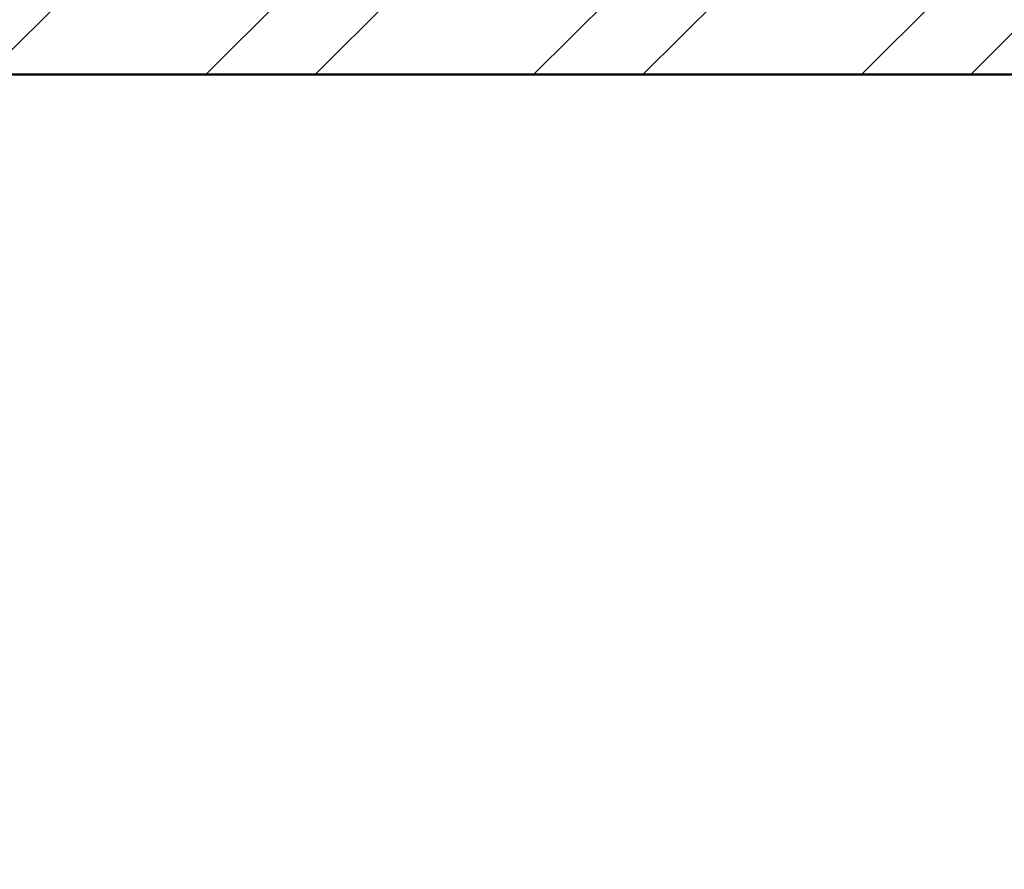
# Model space of a CAD drawing. Units: inches. Extents: x 963 to 2075, y 289 to 2657.
# Tile 77 of 98: x 1426 to 1467, y 2290 to 2325. Entities that reach past the tile are written whole.
import ezdxf

# ---------------------------------------------------------------- set-up
doc = ezdxf.new("R2010")
doc.units = ezdxf.units.IN
doc.layers.add('A-WALL', color=7, linetype='Continuous', lineweight=50)
doc.layers.add('A-WALL-PATT', color=8, linetype='Continuous', lineweight=13)

msp = doc.modelspace()

# ---------------------------------------------------------------- hatches: boundary and pattern name
at = {"layer": 'A-WALL-PATT'}
h = msp.add_hatch(dxfattribs=at)
h.set_pattern_fill('ANSI32', color=256)
h.paths.add_polyline_path([(1296.922, 2558.318), (1203.922, 2558.318), (1203.922, 2493.818), (1191.533, 2493.818), (1191.533, 2489.318), (1211.063, 2489.318), (1211.063, 2492.02), (1211.063, 2493.818), (1208.422, 2493.818), (1208.422, 2553.818), (1292.422, 2553.818), (1292.422, 2538.863), (1296.922, 2538.863)])
h.paths.add_polyline_path([(1442.422, 2558.318), (1349.422, 2558.318), (1349.422, 2538.943), (1353.922, 2538.943), (1353.922, 2553.818), (1437.922, 2553.818), (1437.922, 2493.818), (1434.542, 2493.818), (1434.542, 2489.318), (1448.311, 2489.318), (1448.311, 2491.568), (1448.311, 2493.818), (1442.422, 2493.818)])
h.paths.add_polyline_path([(1415.554, 2491.568), (1415.554, 2493.818), (1340.941, 2493.818), (1340.941, 2489.318), (1371.922, 2489.318), (1371.922, 2378.318), (1367.596, 2378.318), (1367.596, 2373.818), (1371.922, 2373.818), (1371.922, 2355.185), (1376.422, 2355.185), (1376.422, 2489.318), (1415.554, 2489.318)])
h.paths.add_polyline_path([(1304.941, 2491.568), (1304.941, 2493.818), (1296.922, 2493.818), (1296.922, 2514.863), (1292.422, 2514.863), (1292.422, 2493.818), (1232.808, 2493.818), (1232.808, 2489.318), (1256.422, 2489.318), (1256.422, 2327.318), (1253.714, 2327.318), (1253.714, 2322.818), (1328.422, 2322.818), (1328.422, 2331.147), (1323.922, 2331.147), (1323.922, 2327.318), (1260.922, 2327.318), (1260.922, 2373.818), (1323.922, 2373.818), (1323.922, 2357.812), (1328.422, 2357.812), (1328.422, 2373.818), (1346.007, 2373.818), (1346.007, 2376.068), (1346.007, 2378.318), (1260.922, 2378.318), (1260.922, 2489.318), (1304.941, 2489.318)])
h.paths.add_polyline_path([(1226.654, 2327.318), (1124.422, 2327.318), (1124.422, 2347.447), (1119.922, 2347.447), (1119.922, 2322.818), (1163.422, 2322.818), (1163.422, 2305.435), (1165.672, 2305.435), (1167.922, 2305.435), (1167.922, 2322.818), (1226.654, 2322.818), (1226.654, 2325.068)])
h.paths.add_polyline_path([(1095.922, 2489.318), (1124.422, 2489.318), (1131.533, 2489.318), (1131.533, 2491.568), (1131.533, 2493.818), (1119.922, 2493.818), (1091.422, 2493.818), (1091.422, 2417.318), (1095.922, 2417.318), (1119.922, 2417.318), (1119.922, 2407.447), (1124.422, 2407.447), (1124.422, 2421.818), (1095.922, 2421.818)])
h.paths.add_polyline_path([(1512.922, 2558.318), (1508.422, 2558.318), (1508.422, 2493.818), (1503.401, 2493.818), (1503.401, 2489.318), (1508.422, 2489.318), (1508.422, 2327.318), (1376.422, 2327.318), (1376.422, 2330.273), (1371.922, 2330.273), (1371.922, 2298.744), (1376.422, 2298.744), (1376.422, 2322.818), (1508.422, 2322.818), (1508.422, 2165.318), (1504.255, 2165.318), (1504.255, 2160.818), (1508.422, 2160.818), (1508.422, 2108.318), (1512.922, 2108.318), (1512.922, 2160.818), (1516.182, 2160.818), (1516.182, 2163.068), (1516.182, 2165.318), (1512.922, 2165.318), (1512.922, 2322.818), (1644.922, 2322.818), (1644.922, 2298.744), (1649.422, 2298.744), (1649.422, 2322.818), (1649.422, 2330.944), (1647.172, 2330.944), (1644.922, 2330.944), (1644.922, 2327.318), (1512.922, 2327.318), (1512.922, 2489.318), (1516.759, 2489.318), (1516.759, 2491.568), (1516.759, 2493.818), (1512.922, 2493.818)])
h.paths.add_polyline_path([(1671.922, 2558.318), (1578.922, 2558.318), (1578.922, 2493.818), (1573.526, 2493.818), (1573.526, 2489.318), (1586.537, 2489.318), (1586.537, 2491.568), (1586.537, 2493.818), (1583.422, 2493.818), (1583.422, 2553.818), (1667.422, 2553.818), (1667.422, 2541.109), (1671.922, 2541.109)])
h.paths.add_polyline_path([(1681.257, 2493.818), (1671.922, 2493.818), (1671.922, 2517.109), (1667.422, 2517.109), (1667.422, 2493.818), (1610.218, 2493.818), (1610.218, 2489.318), (1644.922, 2489.318), (1644.922, 2357.865), (1649.422, 2357.865), (1649.422, 2373.818), (1652.203, 2373.818), (1652.203, 2375.827), (1652.203, 2378.318), (1649.422, 2378.318), (1649.422, 2489.318), (1681.257, 2489.318), (1681.257, 2491.568)])
h.paths.add_polyline_path([(1821.922, 2558.318), (1728.922, 2558.318), (1728.922, 2541), (1733.422, 2541), (1733.422, 2553.818), (1817.422, 2553.818), (1817.422, 2493.818), (1813.507, 2493.818), (1813.507, 2489.318), (1830.078, 2489.318), (1830.078, 2491.568), (1830.078, 2493.818), (1821.922, 2493.818)])
h.paths.add_polyline_path([(1794.244, 2493.818), (1717.257, 2493.818), (1717.257, 2489.318), (1760.422, 2489.318), (1760.422, 2378.318), (1674.401, 2378.318), (1674.401, 2373.818), (1692.922, 2373.818), (1692.922, 2356.954), (1697.422, 2356.954), (1697.422, 2373.818), (1760.422, 2373.818), (1760.422, 2327.318), (1697.422, 2327.318), (1697.422, 2333.341), (1692.922, 2333.341), (1692.922, 2322.818), (1768.037, 2322.818), (1768.037, 2325.068), (1768.037, 2327.318), (1764.922, 2327.318), (1764.922, 2489.318), (1794.244, 2489.318)])
h.paths.add_polyline_path([(1733.422, 2517), (1728.922, 2517), (1728.922, 2493.818), (1733.422, 2493.818)], flags=17)
h.paths.add_polyline_path([(1929.922, 2493.818), (1890.078, 2493.818), (1890.078, 2489.318), (1896.922, 2489.318), (1925.422, 2489.318), (1925.422, 2421.818), (1896.922, 2421.818), (1896.922, 2408.318), (1901.422, 2408.318), (1901.422, 2417.318), (1925.422, 2417.318), (1929.922, 2417.318)])
h.paths.add_polyline_path([(1901.422, 2348.318), (1896.922, 2348.318), (1896.922, 2327.318), (1800.423, 2327.318), (1800.423, 2322.818), (1853.422, 2322.818), (1853.422, 2309.453), (1857.922, 2309.453), (1857.922, 2322.818), (1901.422, 2322.818)])
h.paths.add_polyline_path([(1857.922, 2249.453), (1853.422, 2249.453), (1853.422, 2214.818), (1686.309, 2214.818), (1686.309, 2210.318), (1853.422, 2210.318), (1853.422, 2202.134), (1857.922, 2202.134), (1857.922, 2210.318)])
h.paths.add_polyline_path([(1857.922, 2142.134), (1853.422, 2142.134), (1853.422, 2115.422), (1841.422, 2115.422), (1841.422, 2088.531), (1841.422, 2046.949), (1845.922, 2046.949), (1845.922, 2110.922), (1905.922, 2110.922), (1905.922, 2092.517), (1910.422, 2092.517), (1910.422, 2115.422), (1857.922, 2115.422)])
h.paths.add_polyline_path([(1532.436, 1482.342), (1573.456, 1482.342), (1573.456, 1501), (1532.436, 1501)], flags=9)
h.paths.add_polyline_path([(1438.658, 1486.302), (1479.678, 1486.302), (1479.678, 1504.96), (1438.658, 1504.96)], flags=9)
h.paths.add_polyline_path([(1411.215, 1365.308), (1659.139, 1365.308), (1659.139, 1402.401), (1411.215, 1402.401)], flags=9)
h.paths.add_polyline_path([(1185.671, 2296.298), (1248.16, 2296.298), (1248.16, 2314.955), (1185.671, 2314.955)], flags=9)
h.paths.add_polyline_path([(1177.31, 2187.35), (1216.15, 2187.35), (1216.15, 2206.007), (1177.31, 2206.007)], flags=9)
h.paths.add_polyline_path([(1295.101, 1602.083), (1328.26, 1602.083), (1328.26, 1620.741), (1295.101, 1620.741)], flags=9)
h.paths.add_polyline_path([(1525.126, 2005.99), (1558.39, 2005.99), (1558.39, 2024.648), (1525.126, 2024.648)], flags=9)
h.paths.add_polyline_path([(1459.606, 1977.125), (1472.195, 1977.125), (1472.195, 1987.429), (1459.606, 1987.429)], flags=9)
h.paths.add_polyline_path([(1467.815, 2053.676), (1480.018, 2053.676), (1480.018, 2063.979), (1467.815, 2063.979)], flags=9)
h.paths.add_polyline_path([(1555.184, 2119.02), (1584.563, 2119.02), (1584.563, 2137.678), (1555.184, 2137.678)], flags=25)
h.paths.add_polyline_path([(1405.389, 2115.291), (1444.478, 2115.291), (1444.478, 2133.948), (1405.389, 2133.948)], flags=25)
h.paths.add_polyline_path([(1698.482, 2004.259), (1727.695, 2004.259), (1727.695, 2022.916), (1698.482, 2022.916)], flags=9)
h.paths.add_polyline_path([(1612.158, 1972.855), (1629.016, 1972.855), (1629.016, 1983.159), (1612.158, 1983.159)], flags=9)
h.paths.add_polyline_path([(1608.289, 2060.036), (1625.147, 2060.036), (1625.147, 2070.34), (1608.289, 2070.34)], flags=9)
h.paths.add_polyline_path([(1527.954, 1684.402), (1566.795, 1684.402), (1566.795, 1703.06), (1527.954, 1703.06)], flags=9)
h.paths.add_polyline_path([(1422.792, 1683.59), (1461.633, 1683.59), (1461.633, 1702.247), (1422.792, 1702.247)], flags=9)
h.paths.add_polyline_path([(1531.262, 1732.459), (1574.015, 1732.459), (1574.015, 1751.116), (1531.262, 1751.116)], flags=9)
h.paths.add_polyline_path([(1402.872, 1732.845), (1439.799, 1732.845), (1439.799, 1751.502), (1402.872, 1751.502)], flags=9)
h.paths.add_polyline_path([(1243.122, 1923.132), (1281.962, 1923.132), (1281.962, 1941.79), (1243.122, 1941.79)], flags=9)
h.paths.add_polyline_path([(1181.752, 1792.268), (1244.241, 1792.268), (1244.241, 1810.926), (1181.752, 1810.926)], flags=9)
h.paths.add_polyline_path([(1265.822, 1670.3), (1316.071, 1670.3), (1316.071, 1688.957), (1265.822, 1688.957)], flags=9)
h.paths.add_polyline_path([(1140.263, 1676.054), (1179.104, 1676.054), (1179.104, 1694.711), (1140.263, 1694.711)], flags=9)
h.paths.add_polyline_path([(1107.49, 1490.889), (1143.374, 1490.889), (1143.374, 1509.546), (1107.49, 1509.546)], flags=9)
h.paths.add_polyline_path([(1217.584, 1483.899), (1246.741, 1483.899), (1246.741, 1502.556), (1217.584, 1502.556)], flags=9)
h.paths.add_polyline_path([(1389.21, 1486.919), (1418.367, 1486.919), (1418.367, 1505.576), (1389.21, 1505.576)], flags=9)
h.paths.add_polyline_path([(1672.208, 1602.083), (1705.366, 1602.083), (1705.366, 1620.741), (1672.208, 1620.741)], flags=9)
h.paths.add_polyline_path([(1752.082, 1522.638), (1781.24, 1522.638), (1781.24, 1541.295), (1752.082, 1541.295)], flags=9)
h.paths.add_polyline_path([(1848.275, 1491.26), (1884.158, 1491.26), (1884.158, 1509.918), (1848.275, 1509.918)], flags=9)
h.paths.add_polyline_path([(1822.47, 1685.62), (1861.31, 1685.62), (1861.31, 1704.278), (1822.47, 1704.278)], flags=9)
h.paths.add_polyline_path([(1713.195, 1672.232), (1763.444, 1672.232), (1763.444, 1690.889), (1713.195, 1690.889)], flags=9)
h.paths.add_polyline_path([(1736.619, 1790.578), (1799.109, 1790.578), (1799.109, 1809.235), (1736.619, 1809.235)], flags=9)
h.paths.add_polyline_path([(1691.491, 1916.355), (1730.332, 1916.355), (1730.332, 1935.013), (1691.491, 1935.013)], flags=9)
h.paths.add_polyline_path([(1764.872, 1973.922), (1794.306, 1973.922), (1794.306, 1992.58), (1764.872, 1992.58)], flags=9)
h.paths.add_polyline_path([(1767.854, 2034.017), (1797.288, 2034.017), (1797.288, 2052.674), (1767.854, 2052.674)], flags=9)
h.paths.add_polyline_path([(1851.593, 2060.331), (1880.751, 2060.331), (1880.751, 2078.989), (1851.593, 2078.989)], flags=25)
h.paths.add_polyline_path([(1688.491, 2086.874), (1727.332, 2086.874), (1727.332, 2105.531), (1688.491, 2105.531)], flags=9)
h.paths.add_polyline_path([(1537.743, 2293.581), (1580.495, 2293.581), (1580.495, 2312.239), (1537.743, 2312.239)], flags=25)
h.paths.add_polyline_path([(1425.587, 2296.109), (1468.34, 2296.109), (1468.34, 2314.766), (1425.587, 2314.766)], flags=25)
h.paths.add_polyline_path([(1278.518, 2004.184), (1307.72, 2004.184), (1307.72, 2022.841), (1278.518, 2022.841)], flags=9)
h.paths.add_polyline_path([(1193.282, 1973.635), (1222.715, 1973.635), (1222.715, 1992.292), (1193.282, 1992.292)], flags=9)
h.paths.add_polyline_path([(1192.411, 2040.577), (1221.845, 2040.577), (1221.845, 2059.234), (1192.411, 2059.234)], flags=9)
h.paths.add_polyline_path([(1130.603, 1951.393), (1159.76, 1951.393), (1159.76, 1970.05), (1130.603, 1970.05)], flags=9)
h.paths.add_polyline_path([(1132.827, 2052.494), (1161.984, 2052.494), (1161.984, 2071.151), (1132.827, 2071.151)], flags=9)
h.paths.add_polyline_path([(1265.128, 2334.619), (1315.377, 2334.619), (1315.377, 2353.277), (1265.128, 2353.277)], flags=25)
h.paths.add_polyline_path([(1136.741, 2330.785), (1175.582, 2330.785), (1175.582, 2349.443), (1136.741, 2349.443)], flags=9)
h.paths.add_polyline_path([(1287.422, 2417.204), (1320.58, 2417.204), (1320.58, 2435.861), (1287.422, 2435.861)], flags=25)
h.paths.add_polyline_path([(1430.988, 2329.159), (1469.828, 2329.159), (1469.828, 2347.816), (1430.988, 2347.816)], flags=25)
h.paths.add_polyline_path([(1525.424, 2329.213), (1564.264, 2329.213), (1564.264, 2347.87), (1525.424, 2347.87)], flags=25)
h.paths.add_polyline_path([(1684.525, 2382.799), (1717.683, 2382.799), (1717.683, 2401.457), (1684.525, 2401.457)], flags=25)
h.paths.add_polyline_path([(1704.805, 2340.293), (1755.054, 2340.293), (1755.054, 2358.95), (1704.805, 2358.95)], flags=25)
h.paths.add_polyline_path([(1694.113, 2287.757), (1756.602, 2287.757), (1756.602, 2306.414), (1694.113, 2306.414)], flags=9)
h.paths.add_polyline_path([(1815.778, 2329.861), (1854.618, 2329.861), (1854.618, 2348.518), (1815.778, 2348.518)], flags=9)
h.paths.add_polyline_path([(1842.873, 2514.256), (1878.756, 2514.256), (1878.756, 2532.914), (1842.873, 2532.914)], flags=9)
h.paths.add_polyline_path([(1769.513, 2531.447), (1798.671, 2531.447), (1798.671, 2550.104), (1769.513, 2550.104)], flags=25)
h.paths.add_polyline_path([(1594.772, 2518.468), (1623.93, 2518.468), (1623.93, 2537.125), (1594.772, 2537.125)], flags=25)
h.paths.add_polyline_path([(1520.723, 2516.185), (1556.606, 2516.185), (1556.606, 2534.842), (1520.723, 2534.842)], flags=25)
h.paths.add_polyline_path([(1464.456, 2516.694), (1500.34, 2516.694), (1500.34, 2535.351), (1464.456, 2535.351)], flags=25)
h.paths.add_polyline_path([(1365.696, 2528.97), (1394.854, 2528.97), (1394.854, 2547.627), (1365.696, 2547.627)], flags=25)
h.paths.add_polyline_path([(1222.838, 2516.231), (1251.995, 2516.231), (1251.995, 2534.889), (1222.838, 2534.889)], flags=25)
h.paths.add_polyline_path([(1104.545, 2509.6), (1140.429, 2509.6), (1140.429, 2528.257), (1104.545, 2528.257)], flags=9)
h = msp.add_hatch(dxfattribs=at)
h.set_pattern_fill('ANSI32', color=256)
h.paths.add_polyline_path([(1335.968, 2212.568), (1335.968, 2214.818), (1167.922, 2214.818), (1167.922, 2245.435), (1163.422, 2245.435), (1163.422, 2210.318), (1163.422, 2194.812), (1167.922, 2194.812), (1167.922, 2210.318), (1335.968, 2210.318)])
h.paths.add_polyline_path([(1532.436, 1482.342), (1573.456, 1482.342), (1573.456, 1501), (1532.436, 1501)], flags=9)
h.paths.add_polyline_path([(1438.658, 1486.302), (1479.678, 1486.302), (1479.678, 1504.96), (1438.658, 1504.96)], flags=9)
h.paths.add_polyline_path([(1411.215, 1365.308), (1659.139, 1365.308), (1659.139, 1402.401), (1411.215, 1402.401)], flags=9)
h.paths.add_polyline_path([(1185.671, 2296.298), (1248.16, 2296.298), (1248.16, 2314.955), (1185.671, 2314.955)], flags=9)
h.paths.add_polyline_path([(1177.31, 2187.35), (1216.15, 2187.35), (1216.15, 2206.007), (1177.31, 2206.007)], flags=9)
h.paths.add_polyline_path([(1295.101, 1602.083), (1328.26, 1602.083), (1328.26, 1620.741), (1295.101, 1620.741)], flags=9)
h.paths.add_polyline_path([(1525.126, 2005.99), (1558.39, 2005.99), (1558.39, 2024.648), (1525.126, 2024.648)], flags=9)
h.paths.add_polyline_path([(1459.606, 1977.125), (1472.195, 1977.125), (1472.195, 1987.429), (1459.606, 1987.429)], flags=9)
h.paths.add_polyline_path([(1467.815, 2053.676), (1480.018, 2053.676), (1480.018, 2063.979), (1467.815, 2063.979)], flags=9)
h.paths.add_polyline_path([(1555.184, 2119.02), (1584.563, 2119.02), (1584.563, 2137.678), (1555.184, 2137.678)], flags=9)
h.paths.add_polyline_path([(1405.389, 2115.291), (1444.478, 2115.291), (1444.478, 2133.948), (1405.389, 2133.948)], flags=9)
h.paths.add_polyline_path([(1698.482, 2004.259), (1727.695, 2004.259), (1727.695, 2022.916), (1698.482, 2022.916)], flags=9)
h.paths.add_polyline_path([(1612.158, 1972.855), (1629.016, 1972.855), (1629.016, 1983.159), (1612.158, 1983.159)], flags=9)
h.paths.add_polyline_path([(1608.289, 2060.036), (1625.147, 2060.036), (1625.147, 2070.34), (1608.289, 2070.34)], flags=9)
h.paths.add_polyline_path([(1527.954, 1684.402), (1566.795, 1684.402), (1566.795, 1703.06), (1527.954, 1703.06)], flags=9)
h.paths.add_polyline_path([(1422.792, 1683.59), (1461.633, 1683.59), (1461.633, 1702.247), (1422.792, 1702.247)], flags=9)
h.paths.add_polyline_path([(1531.262, 1732.459), (1574.015, 1732.459), (1574.015, 1751.116), (1531.262, 1751.116)], flags=9)
h.paths.add_polyline_path([(1402.872, 1732.845), (1439.799, 1732.845), (1439.799, 1751.502), (1402.872, 1751.502)], flags=9)
h.paths.add_polyline_path([(1243.122, 1923.132), (1281.962, 1923.132), (1281.962, 1941.79), (1243.122, 1941.79)], flags=9)
h.paths.add_polyline_path([(1181.752, 1792.268), (1244.241, 1792.268), (1244.241, 1810.926), (1181.752, 1810.926)], flags=9)
h.paths.add_polyline_path([(1265.822, 1670.3), (1316.071, 1670.3), (1316.071, 1688.957), (1265.822, 1688.957)], flags=9)
h.paths.add_polyline_path([(1140.263, 1676.054), (1179.104, 1676.054), (1179.104, 1694.711), (1140.263, 1694.711)], flags=9)
h.paths.add_polyline_path([(1107.49, 1490.889), (1143.374, 1490.889), (1143.374, 1509.546), (1107.49, 1509.546)], flags=9)
h.paths.add_polyline_path([(1217.584, 1483.899), (1246.741, 1483.899), (1246.741, 1502.556), (1217.584, 1502.556)], flags=9)
h.paths.add_polyline_path([(1389.21, 1486.919), (1418.367, 1486.919), (1418.367, 1505.576), (1389.21, 1505.576)], flags=9)
h.paths.add_polyline_path([(1672.208, 1602.083), (1705.366, 1602.083), (1705.366, 1620.741), (1672.208, 1620.741)], flags=9)
h.paths.add_polyline_path([(1752.082, 1522.638), (1781.24, 1522.638), (1781.24, 1541.295), (1752.082, 1541.295)], flags=9)
h.paths.add_polyline_path([(1848.275, 1491.26), (1884.158, 1491.26), (1884.158, 1509.918), (1848.275, 1509.918)], flags=9)
h.paths.add_polyline_path([(1822.47, 1685.62), (1861.31, 1685.62), (1861.31, 1704.278), (1822.47, 1704.278)], flags=9)
h.paths.add_polyline_path([(1713.195, 1672.232), (1763.444, 1672.232), (1763.444, 1690.889), (1713.195, 1690.889)], flags=9)
h.paths.add_polyline_path([(1736.619, 1790.578), (1799.109, 1790.578), (1799.109, 1809.235), (1736.619, 1809.235)], flags=9)
h.paths.add_polyline_path([(1691.491, 1916.355), (1730.332, 1916.355), (1730.332, 1935.013), (1691.491, 1935.013)], flags=9)
h.paths.add_polyline_path([(1764.872, 1973.922), (1794.306, 1973.922), (1794.306, 1992.58), (1764.872, 1992.58)], flags=9)
h.paths.add_polyline_path([(1767.854, 2034.017), (1797.288, 2034.017), (1797.288, 2052.674), (1767.854, 2052.674)], flags=9)
h.paths.add_polyline_path([(1851.593, 2060.331), (1880.751, 2060.331), (1880.751, 2078.989), (1851.593, 2078.989)], flags=9)
h.paths.add_polyline_path([(1688.491, 2086.874), (1727.332, 2086.874), (1727.332, 2105.531), (1688.491, 2105.531)], flags=9)
h.paths.add_polyline_path([(1537.743, 2293.581), (1580.495, 2293.581), (1580.495, 2312.239), (1537.743, 2312.239)], flags=9)
h.paths.add_polyline_path([(1425.587, 2296.109), (1468.34, 2296.109), (1468.34, 2314.766), (1425.587, 2314.766)], flags=9)
h.paths.add_polyline_path([(1278.518, 2004.184), (1307.72, 2004.184), (1307.72, 2022.841), (1278.518, 2022.841)], flags=9)
h.paths.add_polyline_path([(1193.282, 1973.635), (1222.715, 1973.635), (1222.715, 1992.292), (1193.282, 1992.292)], flags=9)
h.paths.add_polyline_path([(1192.411, 2040.577), (1221.845, 2040.577), (1221.845, 2059.234), (1192.411, 2059.234)], flags=9)
h.paths.add_polyline_path([(1130.603, 1951.393), (1159.76, 1951.393), (1159.76, 1970.05), (1130.603, 1970.05)], flags=9)
h.paths.add_polyline_path([(1132.827, 2052.494), (1161.984, 2052.494), (1161.984, 2071.151), (1132.827, 2071.151)], flags=9)
h.paths.add_polyline_path([(1265.128, 2334.619), (1315.377, 2334.619), (1315.377, 2353.277), (1265.128, 2353.277)], flags=9)
h.paths.add_polyline_path([(1136.741, 2330.785), (1175.582, 2330.785), (1175.582, 2349.443), (1136.741, 2349.443)], flags=9)
h.paths.add_polyline_path([(1287.422, 2417.204), (1320.58, 2417.204), (1320.58, 2435.861), (1287.422, 2435.861)], flags=9)
h.paths.add_polyline_path([(1430.988, 2329.159), (1469.828, 2329.159), (1469.828, 2347.816), (1430.988, 2347.816)], flags=9)
h.paths.add_polyline_path([(1525.424, 2329.213), (1564.264, 2329.213), (1564.264, 2347.87), (1525.424, 2347.87)], flags=9)
h.paths.add_polyline_path([(1684.525, 2382.799), (1717.683, 2382.799), (1717.683, 2401.457), (1684.525, 2401.457)], flags=9)
h.paths.add_polyline_path([(1704.805, 2340.293), (1755.054, 2340.293), (1755.054, 2358.95), (1704.805, 2358.95)], flags=9)
h.paths.add_polyline_path([(1694.113, 2287.757), (1756.602, 2287.757), (1756.602, 2306.414), (1694.113, 2306.414)], flags=9)
h.paths.add_polyline_path([(1815.778, 2329.861), (1854.618, 2329.861), (1854.618, 2348.518), (1815.778, 2348.518)], flags=9)
h.paths.add_polyline_path([(1842.873, 2514.256), (1878.756, 2514.256), (1878.756, 2532.914), (1842.873, 2532.914)], flags=9)
h.paths.add_polyline_path([(1769.513, 2531.447), (1798.671, 2531.447), (1798.671, 2550.104), (1769.513, 2550.104)], flags=9)
h.paths.add_polyline_path([(1594.772, 2518.468), (1623.93, 2518.468), (1623.93, 2537.125), (1594.772, 2537.125)], flags=9)
h.paths.add_polyline_path([(1520.723, 2516.185), (1556.606, 2516.185), (1556.606, 2534.842), (1520.723, 2534.842)], flags=9)
h.paths.add_polyline_path([(1464.456, 2516.694), (1500.34, 2516.694), (1500.34, 2535.351), (1464.456, 2535.351)], flags=9)
h.paths.add_polyline_path([(1365.696, 2528.97), (1394.854, 2528.97), (1394.854, 2547.627), (1365.696, 2547.627)], flags=9)
h.paths.add_polyline_path([(1222.838, 2516.231), (1251.995, 2516.231), (1251.995, 2534.889), (1222.838, 2534.889)], flags=9)
h.paths.add_polyline_path([(1104.545, 2509.6), (1140.429, 2509.6), (1140.429, 2528.257), (1104.545, 2528.257)], flags=9)

# ---------------------------------------------------------------- linework, layer by layer
at = {"layer": 'A-WALL'}
msp.add_line((1376.422, 2322.818), (1508.422, 2322.818), dxfattribs=at)

doc.saveas('drawing.dxf')
